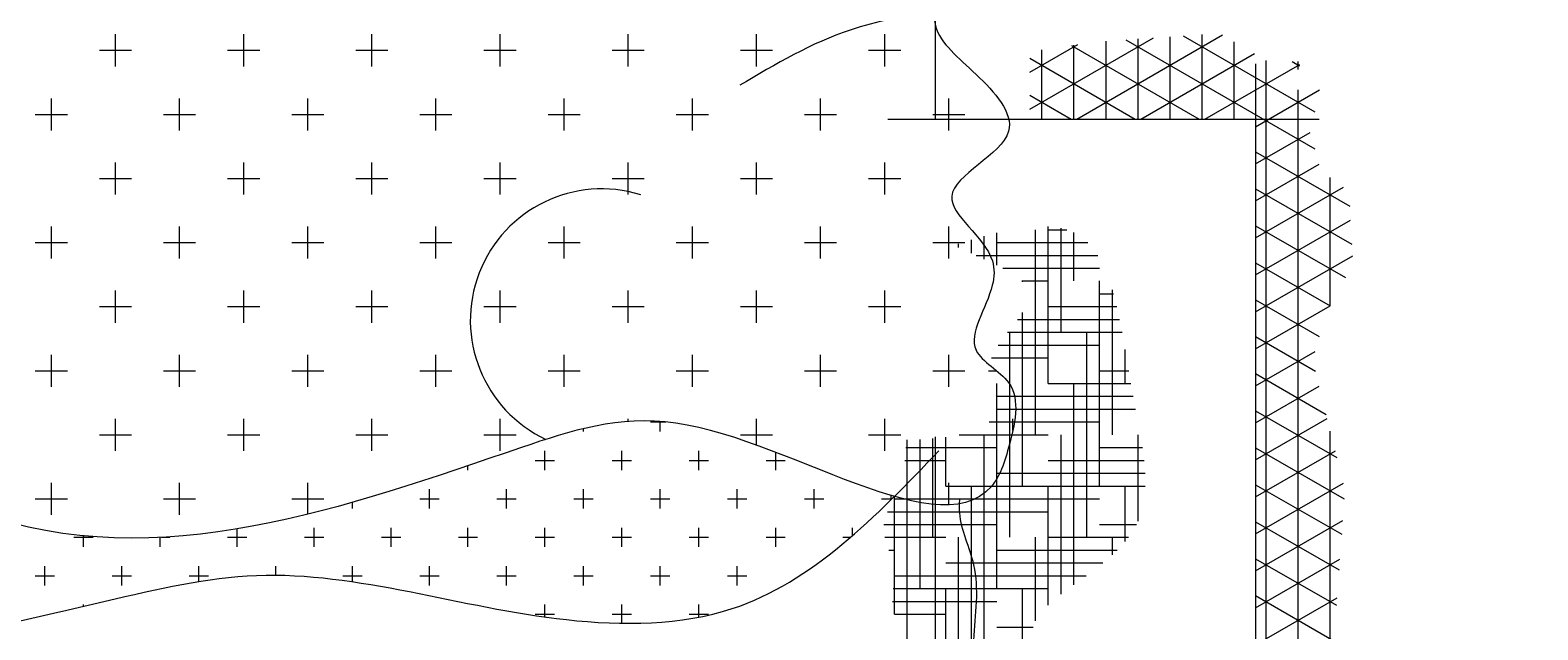
# Model space of a CAD drawing. Units: inches. Extents: x 3731 to 4318, y 1310 to 2388.
# Tile 28 of 57: x 3894 to 3954, y 1882 to 1906. Entities that reach past the tile are written whole.
import ezdxf

# ---------------------------------------------------------------- set-up
doc = ezdxf.new("R2010")
doc.units = ezdxf.units.IN
doc.layers.add('A-ANNO-DIMS', color=2, linetype='Continuous', lineweight=18)
doc.layers.add('A-FURN', color=8, linetype='Continuous', lineweight=13)
doc.styles.get("Standard").update_dxf_attribs({"font": 'arial.ttf'})
doc.dimstyles.get("Standard").update_dxf_attribs({"dimtxt": 0.18, "dimasz": 0.18, "dimexe": 0.18, "dimexo": 0.0625, "dimgap": 0.09, "dimtad": 0, "dimtih": 1, "dimtoh": 1, "dimdec": 4, "dimzin": 0, "dimdsep": 46, "dimtxsty": 'Standard', "dimcen": 0.09, "dimadec": 0, "dimazin": 0, "dimtfac": 1, "dimtdec": 4, "dimtofl": 0, "dimtmove": 0, "dimatfit": 3, "dimfxl": 1, "dimtolj": 1, "dimtzin": 0, "dimarcsym": 0})

# ---------------------------------------------------------------- blocks, each defined once
blk = doc.blocks.new('A$C200C7901')
for p, q in [((2, 1.6055), (2, 2.3334)), ((2.3121, 1.6596), (2.3121, 0.0201)), ((1.9533, 1.6055), (2.3741, 1.6055)), ((1.9533, 1.6055), (2.3741, 1.6055)), ((2, 0.2957), (2, 1.2957)), ((2.0224, 0.9977), (2.0224, 1.1977)), ((2.0224, 0.9977), (2.0224, 1.1977))]:
    blk.add_line(p, q)
at = {"linetype": 'ByBlock'}
for p, q in [((1.2004, 1.657), (1.2004, 1.6883)), ((1.2004, 1.657), (1.2004, 1.6883)), ((1.3254, 1.657), (1.3254, 1.6883)), ((1.3254, 1.657), (1.3254, 1.6883)), ((1.4504, 1.657), (1.4504, 1.6883)), ((1.4504, 1.657), (1.4504, 1.6883)), ((1.5754, 1.657), (1.5754, 1.6883)), ((1.5754, 1.657), (1.5754, 1.6883)), ((1.7004, 1.657), (1.7004, 1.6883)), ((1.7004, 1.657), (1.7004, 1.6883)), ((1.8254, 1.657), (1.8254, 1.6883)), ((1.8254, 1.657), (1.8254, 1.6883)), ((1.9504, 1.657), (1.9504, 1.6883)), ((1.9504, 1.657), (1.9504, 1.6883)), ((2.0919, 1.6152), (2.2125, 1.6848)), ((2.0919, 1.6152), (2.2125, 1.6848)), ((2.0919, 1.6513), (2.1386, 1.6782)), ((2.0919, 1.6513), (2.1386, 1.6782)), ((2.1327, 1.6773), (2.2571, 1.6055)), ((2.1327, 1.6773), (2.2571, 1.6055)), ((2.1349, 1.6055), (2.1349, 1.6777)), ((2.1349, 1.6055), (2.1349, 1.6777)), ((2.1377, 1.6055), (2.2798, 1.6876)), ((2.1377, 1.6055), (2.2798, 1.6876)), ((2.1662, 1.6055), (2.1662, 1.6817)), ((2.1662, 1.6055), (2.1662, 1.6817)), ((2.1854, 1.683), (2.3697, 1.5766)), ((2.1854, 1.683), (2.3697, 1.5766)), ((2.1974, 1.6055), (2.1974, 1.6838)), ((2.1974, 1.6055), (2.1974, 1.6838)), ((2.2287, 1.6055), (2.2287, 1.6859)), ((2.2287, 1.6055), (2.2287, 1.6859)), ((2.2414, 1.6868), (2.3699, 1.6126)), ((2.2414, 1.6868), (2.3699, 1.6126)), ((2.2599, 1.6055), (2.2599, 1.688)), ((2.2599, 1.6055), (2.2599, 1.688)), ((2.2912, 1.6055), (2.2912, 1.6809)), ((2.2912, 1.6055), (2.2912, 1.6809)), ((1.1847, 1.6727), (1.216, 1.6727)), ((1.1847, 1.6727), (1.216, 1.6727)), ((1.3097, 1.6727), (1.341, 1.6727)), ((1.3097, 1.6727), (1.341, 1.6727)), ((1.4347, 1.6727), (1.466, 1.6727)), ((1.4347, 1.6727), (1.466, 1.6727)), ((1.5597, 1.6727), (1.591, 1.6727)), ((1.5597, 1.6727), (1.591, 1.6727)), ((1.6847, 1.6727), (1.716, 1.6727)), ((1.6847, 1.6727), (1.716, 1.6727)), ((1.8097, 1.6727), (1.841, 1.6727)), ((1.8097, 1.6727), (1.841, 1.6727)), ((1.9347, 1.6727), (1.966, 1.6727)), ((1.9347, 1.6727), (1.966, 1.6727)), ((2.0919, 1.6649), (2.1946, 1.6055)), ((2.0919, 1.6649), (2.1946, 1.6055)), ((2.1037, 1.6055), (2.1037, 1.673)), ((2.1037, 1.6055), (2.1037, 1.673)), ((2.2002, 1.6055), (2.3109, 1.6694)), ((2.2002, 1.6055), (2.3109, 1.6694)), ((2.3224, 0.0468), (2.3224, 1.6627)), ((2.3224, 0.0468), (2.3224, 1.6627)), ((2.3476, 1.6616), (2.3547, 1.6575)), ((2.3476, 1.6616), (2.3547, 1.6575)), ((2.3537, 1.6539), (2.3537, 1.6616)), ((2.3537, 1.6539), (2.3537, 1.6616)), ((2.2627, 1.6055), (2.3551, 1.6589)), ((2.2627, 1.6055), (2.3551, 1.6589)), ((2.3121, 1.598), (2.3745, 1.634)), ((2.3121, 1.598), (2.3745, 1.634)), ((2.3537, 0.0056), (2.3537, 1.634)), ((2.3537, 0.0056), (2.3537, 1.634)), ((1.1379, 1.5945), (1.1379, 1.6258)), ((1.1379, 1.5945), (1.1379, 1.6258)), ((1.2629, 1.5945), (1.2629, 1.6258)), ((1.2629, 1.5945), (1.2629, 1.6258)), ((1.3879, 1.5945), (1.3879, 1.6258)), ((1.3879, 1.5945), (1.3879, 1.6258)), ((1.5129, 1.5945), (1.5129, 1.6258)), ((1.5129, 1.5945), (1.5129, 1.6258)), ((1.6379, 1.5945), (1.6379, 1.6258)), ((1.6379, 1.5945), (1.6379, 1.6258)), ((1.7629, 1.5945), (1.7629, 1.6258)), ((1.7629, 1.5945), (1.7629, 1.6258)), ((1.8879, 1.5945), (1.8879, 1.6258)), ((1.8879, 1.5945), (1.8879, 1.6258)), ((2.0129, 1.5945), (2.0129, 1.6258)), ((2.0129, 1.5945), (2.0129, 1.6258)), ((2.0919, 1.6288), (2.1321, 1.6055)), ((2.0919, 1.6288), (2.1321, 1.6055)), ((1.1222, 1.6102), (1.1535, 1.6102)), ((1.1222, 1.6102), (1.1535, 1.6102)), ((1.2472, 1.6102), (1.2785, 1.6102)), ((1.2472, 1.6102), (1.2785, 1.6102)), ((1.3722, 1.6102), (1.4035, 1.6102)), ((1.3722, 1.6102), (1.4035, 1.6102)), ((1.4972, 1.6102), (1.5285, 1.6102)), ((1.4972, 1.6102), (1.5285, 1.6102)), ((1.6222, 1.6102), (1.6535, 1.6102)), ((1.6222, 1.6102), (1.6535, 1.6102)), ((1.7472, 1.6102), (1.7785, 1.6102)), ((1.7472, 1.6102), (1.7785, 1.6102)), ((1.8722, 1.6102), (1.9035, 1.6102)), ((1.8722, 1.6102), (1.9035, 1.6102)), ((1.9972, 1.6102), (2.0285, 1.6102)), ((1.9972, 1.6102), (2.0285, 1.6102)), ((2.3121, 1.5619), (2.3654, 1.5926)), ((2.3121, 1.5619), (2.3654, 1.5926)), ((2.3121, 1.5738), (2.404, 1.5208)), ((2.3121, 1.5738), (2.404, 1.5208)), ((1.2004, 1.532), (1.2004, 1.5633)), ((1.2004, 1.532), (1.2004, 1.5633)), ((1.3254, 1.532), (1.3254, 1.5633)), ((1.3254, 1.532), (1.3254, 1.5633)), ((1.4504, 1.532), (1.4504, 1.5633)), ((1.4504, 1.532), (1.4504, 1.5633)), ((1.5754, 1.532), (1.5754, 1.5633)), ((1.5754, 1.532), (1.5754, 1.5633)), ((1.7004, 1.532), (1.7004, 1.5633)), ((1.7004, 1.532), (1.7004, 1.5633)), ((1.8254, 1.532), (1.8254, 1.5633)), ((1.8254, 1.532), (1.8254, 1.5633)), ((1.9504, 1.532), (1.9504, 1.5633)), ((1.9504, 1.532), (1.9504, 1.5633)), ((2.3121, 1.5258), (2.3739, 1.5615)), ((2.3121, 1.5258), (2.3739, 1.5615)), ((1.1847, 1.5477), (1.216, 1.5477)), ((1.1847, 1.5477), (1.216, 1.5477)), ((1.3097, 1.5477), (1.341, 1.5477)), ((1.3097, 1.5477), (1.341, 1.5477)), ((1.4347, 1.5477), (1.466, 1.5477)), ((1.4347, 1.5477), (1.466, 1.5477)), ((1.5597, 1.5477), (1.591, 1.5477)), ((1.5597, 1.5477), (1.591, 1.5477)), ((1.6847, 1.5477), (1.716, 1.5477)), ((1.6847, 1.5477), (1.716, 1.5477)), ((1.8097, 1.5477), (1.841, 1.5477)), ((1.8097, 1.5477), (1.841, 1.5477)), ((1.9347, 1.5477), (1.966, 1.5477)), ((1.9347, 1.5477), (1.966, 1.5477)), ((2.3849, 1.4236), (2.3849, 1.5486)), ((2.3849, 1.4236), (2.3849, 1.5486)), ((2.3121, 1.4897), (2.3979, 1.5393)), ((2.3121, 1.4897), (2.3979, 1.5393)), ((2.3121, 1.5377), (2.406, 1.4835)), ((2.3121, 1.5377), (2.406, 1.4835)), ((1.1379, 1.4695), (1.1379, 1.5008)), ((1.1379, 1.4695), (1.1379, 1.5008)), ((1.2629, 1.4695), (1.2629, 1.5008)), ((1.2629, 1.4695), (1.2629, 1.5008)), ((1.3879, 1.4695), (1.3879, 1.5008)), ((1.3879, 1.4695), (1.3879, 1.5008)), ((1.5129, 1.4695), (1.5129, 1.5008)), ((1.5129, 1.4695), (1.5129, 1.5008)), ((1.6379, 1.4695), (1.6379, 1.5008)), ((1.6379, 1.4695), (1.6379, 1.5008)), ((1.7629, 1.4695), (1.7629, 1.5008)), ((1.7629, 1.4695), (1.7629, 1.5008)), ((1.8879, 1.4695), (1.8879, 1.5008)), ((1.8879, 1.4695), (1.8879, 1.5008)), ((2.0129, 1.4695), (2.0129, 1.5008)), ((2.0129, 1.4695), (2.0129, 1.5008)), ((2.1099, 1.3477), (2.1099, 1.5009)), ((2.1099, 1.3477), (2.1099, 1.5009)), ((2.3121, 1.4537), (2.4047, 1.5071)), ((2.3121, 1.4537), (2.4047, 1.5071)), ((2.3121, 1.5016), (2.3997, 1.4511)), ((2.3121, 1.5016), (2.3997, 1.4511)), ((1.1222, 1.4852), (1.1535, 1.4852)), ((1.1222, 1.4852), (1.1535, 1.4852)), ((1.2472, 1.4852), (1.2785, 1.4852)), ((1.2472, 1.4852), (1.2785, 1.4852)), ((1.3722, 1.4852), (1.4035, 1.4852)), ((1.3722, 1.4852), (1.4035, 1.4852)), ((1.4972, 1.4852), (1.5285, 1.4852)), ((1.4972, 1.4852), (1.5285, 1.4852)), ((1.6222, 1.4852), (1.6535, 1.4852)), ((1.6222, 1.4852), (1.6535, 1.4852)), ((1.7472, 1.4852), (1.7785, 1.4852)), ((1.7472, 1.4852), (1.7785, 1.4852)), ((1.8722, 1.4852), (1.9035, 1.4852)), ((1.8722, 1.4852), (1.9035, 1.4852)), ((1.9972, 1.4852), (2.0285, 1.4852)), ((1.9972, 1.4852), (2.0285, 1.4852)), ((2.0349, 1.4748), (2.0349, 1.4879)), ((2.0349, 1.4748), (2.0349, 1.4879)), ((2.0474, 1.4691), (2.0474, 1.4915)), ((2.0474, 1.4691), (2.0474, 1.4915)), ((2.0599, 1.4631), (2.0599, 1.4948)), ((2.0599, 1.4631), (2.0599, 1.4948)), ((2.0599, 1.4852), (2.1484, 1.4852)), ((2.0599, 1.4852), (2.1484, 1.4852)), ((2.0974, 1.2977), (2.0974, 1.4977)), ((2.0974, 1.2977), (2.0974, 1.4977)), ((2.1099, 1.4977), (2.1279, 1.4977)), ((2.1099, 1.4977), (2.1279, 1.4977)), ((2.1224, 1.3977), (2.1224, 1.4992)), ((2.1224, 1.3977), (2.1224, 1.4992)), ((2.1349, 1.4477), (2.1349, 1.4949)), ((2.1349, 1.4477), (2.1349, 1.4949)), ((2.0224, 1.4805), (2.0224, 1.4839)), ((2.0224, 1.4805), (2.0224, 1.4839)), ((2.0397, 1.4727), (2.1581, 1.4727)), ((2.0397, 1.4727), (2.1581, 1.4727)), ((2.3121, 1.4176), (2.4067, 1.4721)), ((2.3121, 1.4176), (2.4067, 1.4721)), ((2.0656, 1.4602), (2.1599, 1.4602)), ((2.0656, 1.4602), (2.1599, 1.4602)), ((2.3121, 1.4655), (2.3849, 1.4235)), ((2.3121, 1.4655), (2.3849, 1.4235)), ((2.084, 1.4477), (2.1099, 1.4477)), ((2.084, 1.4477), (2.1099, 1.4477)), ((2.0849, 1.4468), (2.0849, 1.4477)), ((2.0849, 1.4468), (2.0849, 1.4477)), ((2.1599, 1.2477), (2.1599, 1.4477)), ((2.1599, 1.2477), (2.1599, 1.4477)), ((1.2004, 1.407), (1.2004, 1.4383)), ((1.2004, 1.407), (1.2004, 1.4383)), ((1.3254, 1.407), (1.3254, 1.4383)), ((1.3254, 1.407), (1.3254, 1.4383)), ((1.4504, 1.407), (1.4504, 1.4383)), ((1.4504, 1.407), (1.4504, 1.4383)), ((1.5754, 1.407), (1.5754, 1.4383)), ((1.5754, 1.407), (1.5754, 1.4383)), ((1.7004, 1.407), (1.7004, 1.4383)), ((1.7004, 1.407), (1.7004, 1.4383)), ((1.8254, 1.407), (1.8254, 1.4383)), ((1.8254, 1.407), (1.8254, 1.4383)), ((1.9504, 1.407), (1.9504, 1.4383)), ((1.9504, 1.407), (1.9504, 1.4383)), ((2.1599, 1.4352), (2.1735, 1.4352)), ((2.1599, 1.4352), (2.1735, 1.4352)), ((2.1724, 1.2977), (2.1724, 1.439)), ((2.1724, 1.2977), (2.1724, 1.439)), ((2.3121, 1.4294), (2.3741, 1.3937)), ((2.3121, 1.4294), (2.3741, 1.3937)), ((1.1847, 1.4227), (1.216, 1.4227)), ((1.1847, 1.4227), (1.216, 1.4227)), ((1.3097, 1.4227), (1.341, 1.4227)), ((1.3097, 1.4227), (1.341, 1.4227)), ((1.4347, 1.4227), (1.466, 1.4227)), ((1.4347, 1.4227), (1.466, 1.4227)), ((1.5597, 1.4227), (1.591, 1.4227)), ((1.5597, 1.4227), (1.591, 1.4227)), ((1.6847, 1.4227), (1.716, 1.4227)), ((1.6847, 1.4227), (1.716, 1.4227)), ((1.8097, 1.4227), (1.841, 1.4227)), ((1.8097, 1.4227), (1.841, 1.4227)), ((1.9347, 1.4227), (1.966, 1.4227)), ((1.9347, 1.4227), (1.966, 1.4227)), ((2.0849, 1.2477), (2.0849, 1.4171)), ((2.0849, 1.2477), (2.0849, 1.4171)), ((2.1099, 1.4227), (2.1767, 1.4227)), ((2.1099, 1.4227), (2.1767, 1.4227)), ((2.3121, 1.3815), (2.3848, 1.4235)), ((2.3121, 1.3815), (2.3848, 1.4235)), ((2.0703, 1.3977), (2.1819, 1.3977)), ((2.0703, 1.3977), (2.1819, 1.3977)), ((2.0724, 1.1977), (2.0724, 1.3977)), ((2.0724, 1.1977), (2.0724, 1.3977)), ((2.08, 1.4102), (2.1795, 1.4102)), ((2.08, 1.4102), (2.1795, 1.4102)), ((2.1474, 1.1977), (2.1474, 1.3977)), ((2.1474, 1.1977), (2.1474, 1.3977)), ((2.0612, 1.3852), (2.1599, 1.3852)), ((2.0612, 1.3852), (2.1599, 1.3852)), ((2.3121, 1.3934), (2.3703, 1.3598)), ((2.3121, 1.3934), (2.3703, 1.3598)), ((1.1379, 1.3445), (1.1379, 1.3758)), ((1.1379, 1.3445), (1.1379, 1.3758)), ((1.2629, 1.3445), (1.2629, 1.3758)), ((1.2629, 1.3445), (1.2629, 1.3758)), ((1.3879, 1.3445), (1.3879, 1.3758)), ((1.3879, 1.3445), (1.3879, 1.3758)), ((1.5129, 1.3445), (1.5129, 1.3758)), ((1.5129, 1.3445), (1.5129, 1.3758)), ((1.6379, 1.3445), (1.6379, 1.3758)), ((1.6379, 1.3445), (1.6379, 1.3758)), ((1.7629, 1.3445), (1.7629, 1.3758)), ((1.7629, 1.3445), (1.7629, 1.3758)), ((1.8879, 1.3445), (1.8879, 1.3758)), ((1.8879, 1.3445), (1.8879, 1.3758)), ((2.0129, 1.3445), (2.0129, 1.3758)), ((2.0129, 1.3445), (2.0129, 1.3758)), ((2.0545, 1.3727), (2.1099, 1.3727)), ((2.0545, 1.3727), (2.1099, 1.3727)), ((2.1849, 1.3477), (2.1849, 1.3808)), ((2.1849, 1.3477), (2.1849, 1.3808)), ((2.3121, 1.3454), (2.37, 1.3788)), ((2.3121, 1.3454), (2.37, 1.3788)), ((1.1222, 1.3602), (1.1535, 1.3602)), ((1.1222, 1.3602), (1.1535, 1.3602)), ((1.2472, 1.3602), (1.2785, 1.3602)), ((1.2472, 1.3602), (1.2785, 1.3602)), ((1.3722, 1.3602), (1.4035, 1.3602)), ((1.3722, 1.3602), (1.4035, 1.3602)), ((1.4972, 1.3602), (1.5285, 1.3602)), ((1.4972, 1.3602), (1.5285, 1.3602)), ((1.6222, 1.3602), (1.6535, 1.3602)), ((1.6222, 1.3602), (1.6535, 1.3602)), ((1.7472, 1.3602), (1.7785, 1.3602)), ((1.7472, 1.3602), (1.7785, 1.3602)), ((1.8722, 1.3602), (1.9035, 1.3602)), ((1.8722, 1.3602), (1.9035, 1.3602)), ((1.9972, 1.3602), (2.0285, 1.3602)), ((1.9972, 1.3602), (2.0285, 1.3602)), ((2.0515, 1.3602), (2.0599, 1.3602)), ((2.0515, 1.3602), (2.0599, 1.3602)), ((2.1599, 1.3602), (2.1883, 1.3602)), ((2.1599, 1.3602), (2.1883, 1.3602)), ((2.3121, 1.3573), (2.3808, 1.3176)), ((2.3121, 1.3573), (2.3808, 1.3176)), ((2.0599, 1.1477), (2.0599, 1.3477)), ((2.0599, 1.1477), (2.0599, 1.3477)), ((2.1099, 1.3477), (2.1904, 1.3477)), ((2.1099, 1.3477), (2.1904, 1.3477)), ((2.1349, 1.1515), (2.1349, 1.3477)), ((2.1349, 1.1515), (2.1349, 1.3477)), ((2.3121, 1.3093), (2.374, 1.345)), ((2.3121, 1.3093), (2.374, 1.345)), ((2.0599, 1.3352), (2.1926, 1.3352)), ((2.0599, 1.3352), (2.1926, 1.3352)), ((1.2004, 1.282), (1.2004, 1.3133)), ((1.2004, 1.282), (1.2004, 1.3133)), ((1.3254, 1.282), (1.3254, 1.3133)), ((1.3254, 1.282), (1.3254, 1.3133)), ((1.4504, 1.282), (1.4504, 1.3133)), ((1.4504, 1.282), (1.4504, 1.3133)), ((1.5754, 1.282), (1.5754, 1.3133)), ((1.5754, 1.282), (1.5754, 1.3133)), ((1.7004, 1.3106), (1.7004, 1.3133)), ((1.7004, 1.3106), (1.7004, 1.3133)), ((1.7222, 1.3102), (1.7369, 1.3102)), ((1.7222, 1.3102), (1.7369, 1.3102)), ((1.7316, 1.3008), (1.7316, 1.3106)), ((1.7316, 1.3008), (1.7316, 1.3106)), ((1.8254, 1.2876), (1.8254, 1.3133)), ((1.8254, 1.2876), (1.8254, 1.3133)), ((1.9504, 1.282), (1.9504, 1.3133)), ((1.9504, 1.282), (1.9504, 1.3133)), ((2.0524, 1.3102), (2.1599, 1.3102)), ((2.0524, 1.3102), (2.1599, 1.3102)), ((2.0594, 1.3227), (2.195, 1.3227)), ((2.0594, 1.3227), (2.195, 1.3227)), ((2.0754, 1.3017), (2.0754, 1.3133)), ((2.0754, 1.3017), (2.0754, 1.3133)), ((2.3121, 1.3212), (2.3914, 1.2754)), ((2.3121, 1.3212), (2.3914, 1.2754)), ((2.3121, 1.2732), (2.3819, 1.3135)), ((2.3121, 1.2732), (2.3819, 1.3135)), ((1.1847, 1.2977), (1.216, 1.2977)), ((1.1847, 1.2977), (1.216, 1.2977)), ((1.3097, 1.2977), (1.341, 1.2977)), ((1.3097, 1.2977), (1.341, 1.2977)), ((1.4347, 1.2977), (1.466, 1.2977)), ((1.4347, 1.2977), (1.466, 1.2977)), ((1.5597, 1.2977), (1.591, 1.2977)), ((1.5597, 1.2977), (1.591, 1.2977)), ((1.6566, 1.3008), (1.6566, 1.3036)), ((1.6566, 1.3008), (1.6566, 1.3036)), ((1.8097, 1.2977), (1.841, 1.2977)), ((1.8097, 1.2977), (1.841, 1.2977)), ((1.9347, 1.2977), (1.966, 1.2977)), ((1.9347, 1.2977), (1.966, 1.2977)), ((1.9974, 1.1977), (1.9974, 1.2939)), ((1.9974, 1.1977), (1.9974, 1.2939)), ((2.0099, 1.2477), (2.0099, 1.2953)), ((2.0099, 1.2477), (2.0099, 1.2953)), ((2.023, 1.2977), (2.1099, 1.2977)), ((2.023, 1.2977), (2.1099, 1.2977)), ((2.0474, 1.0977), (2.0474, 1.2977)), ((2.0474, 1.0977), (2.0474, 1.2977)), ((2.0597, 1.2977), (2.0744, 1.2977)), ((2.0597, 1.2977), (2.0744, 1.2977)), ((2.1224, 1.1421), (2.1224, 1.2977)), ((2.1224, 1.1421), (2.1224, 1.2977)), ((2.1974, 1.2135), (2.1974, 1.2977)), ((2.1974, 1.2135), (2.1974, 1.2977)), ((2.3849, 1.0607), (2.3849, 1.3013)), ((2.3849, 1.0607), (2.3849, 1.3013)), ((1.6191, 1.2633), (1.6191, 1.282)), ((1.6191, 1.2633), (1.6191, 1.282)), ((1.6941, 1.2633), (1.6941, 1.282)), ((1.6941, 1.2633), (1.6941, 1.282)), ((1.7691, 1.2633), (1.7691, 1.282)), ((1.7691, 1.2633), (1.7691, 1.282)), ((1.8441, 1.2633), (1.8441, 1.2806)), ((1.8441, 1.2633), (1.8441, 1.2806)), ((1.9711, 1.2852), (2.0599, 1.2852)), ((1.9711, 1.2852), (2.0599, 1.2852)), ((1.9724, 1.0977), (1.9724, 1.2927)), ((1.9724, 1.0977), (1.9724, 1.2927)), ((1.9849, 1.1477), (1.9849, 1.293)), ((1.9849, 1.1477), (1.9849, 1.293)), ((2.1599, 1.2852), (2.2018, 1.2852)), ((2.1599, 1.2852), (2.2018, 1.2852)), ((2.3121, 1.2851), (2.3985, 1.2352)), ((2.3121, 1.2851), (2.3985, 1.2352)), ((2.3121, 1.2371), (2.3898, 1.282)), ((2.3121, 1.2371), (2.3898, 1.282)), ((1.5441, 1.2633), (1.5441, 1.2675)), ((1.5441, 1.2633), (1.5441, 1.2675)), ((1.6097, 1.2727), (1.6285, 1.2727)), ((1.6097, 1.2727), (1.6285, 1.2727)), ((1.6847, 1.2727), (1.7035, 1.2727)), ((1.6847, 1.2727), (1.7035, 1.2727)), ((1.7597, 1.2727), (1.7785, 1.2727)), ((1.7597, 1.2727), (1.7785, 1.2727)), ((1.8347, 1.2727), (1.8535, 1.2727)), ((1.8347, 1.2727), (1.8535, 1.2727)), ((1.97, 1.2727), (2.0099, 1.2727)), ((1.97, 1.2727), (2.0099, 1.2727)), ((2.1099, 1.2727), (2.2034, 1.2727)), ((2.1099, 1.2727), (2.2034, 1.2727)), ((1.1379, 1.2195), (1.1379, 1.2508)), ((1.1379, 1.2195), (1.1379, 1.2508)), ((1.2629, 1.2195), (1.2629, 1.2508)), ((1.2629, 1.2195), (1.2629, 1.2508)), ((1.3879, 1.2202), (1.3879, 1.2508)), ((1.3879, 1.2202), (1.3879, 1.2508)), ((2.0129, 1.2293), (2.0129, 1.2508)), ((2.0129, 1.2293), (2.0129, 1.2508)), ((2.0599, 1.2602), (2.2044, 1.2602)), ((2.0599, 1.2602), (2.2044, 1.2602)), ((2.3121, 1.2011), (2.3976, 1.2504)), ((2.3121, 1.2011), (2.3976, 1.2504)), ((1.1222, 1.2352), (1.1535, 1.2352)), ((1.1222, 1.2352), (1.1535, 1.2352)), ((1.2472, 1.2352), (1.2785, 1.2352)), ((1.2472, 1.2352), (1.2785, 1.2352)), ((1.3722, 1.2352), (1.4035, 1.2352)), ((1.3722, 1.2352), (1.4035, 1.2352)), ((1.4972, 1.2352), (1.516, 1.2352)), ((1.4972, 1.2352), (1.516, 1.2352)), ((1.5066, 1.2258), (1.5066, 1.2445)), ((1.5066, 1.2258), (1.5066, 1.2445)), ((1.5722, 1.2352), (1.591, 1.2352)), ((1.5722, 1.2352), (1.591, 1.2352)), ((1.5816, 1.2258), (1.5816, 1.2445)), ((1.5816, 1.2258), (1.5816, 1.2445)), ((1.6472, 1.2352), (1.666, 1.2352)), ((1.6472, 1.2352), (1.666, 1.2352)), ((1.6566, 1.2258), (1.6566, 1.2445)), ((1.6566, 1.2258), (1.6566, 1.2445)), ((1.7222, 1.2352), (1.741, 1.2352)), ((1.7222, 1.2352), (1.741, 1.2352)), ((1.7316, 1.2258), (1.7316, 1.2445)), ((1.7316, 1.2258), (1.7316, 1.2445)), ((1.7972, 1.2352), (1.816, 1.2352)), ((1.7972, 1.2352), (1.816, 1.2352)), ((1.8066, 1.2258), (1.8066, 1.2445)), ((1.8066, 1.2258), (1.8066, 1.2445)), ((1.8722, 1.2352), (1.891, 1.2352)), ((1.8722, 1.2352), (1.891, 1.2352)), ((1.8816, 1.2258), (1.8816, 1.2445)), ((1.8816, 1.2258), (1.8816, 1.2445)), ((1.9472, 1.2352), (1.9574, 1.2352)), ((1.9472, 1.2352), (1.9574, 1.2352)), ((1.9566, 1.2344), (1.9566, 1.2385)), ((1.9566, 1.2344), (1.9566, 1.2385)), ((1.9599, 1.1228), (1.9599, 1.2373)), ((1.9599, 1.1228), (1.9599, 1.2373)), ((1.9599, 1.2352), (2.1599, 1.2352)), ((1.9599, 1.2352), (2.1599, 1.2352)), ((2, 1.2352), (2.0285, 1.2352)), ((2, 1.2352), (2.0285, 1.2352)), ((2.0099, 1.2477), (2.2045, 1.2477)), ((2.0099, 1.2477), (2.2045, 1.2477)), ((2.0349, 1.0477), (2.0349, 1.2477)), ((2.0349, 1.0477), (2.0349, 1.2477)), ((2.1099, 1.1315), (2.1099, 1.2477)), ((2.1099, 1.1315), (2.1099, 1.2477)), ((2.1849, 1.1935), (2.1849, 1.2477)), ((2.1849, 1.1935), (2.1849, 1.2477)), ((2.3121, 1.249), (2.396, 1.2006)), ((2.3121, 1.249), (2.396, 1.2006)), ((1.4316, 1.2258), (1.4316, 1.2318)), ((1.4316, 1.2258), (1.4316, 1.2318)), ((1.953, 1.2227), (2.1099, 1.2227)), ((1.953, 1.2227), (2.1099, 1.2227)), ((1.3191, 1.1883), (1.3191, 1.2059)), ((1.3191, 1.1883), (1.3191, 1.2059)), ((1.3941, 1.1883), (1.3941, 1.207)), ((1.3941, 1.1883), (1.3941, 1.207)), ((1.4691, 1.1883), (1.4691, 1.207)), ((1.4691, 1.1883), (1.4691, 1.207)), ((1.5441, 1.1883), (1.5441, 1.207)), ((1.5441, 1.1883), (1.5441, 1.207)), ((1.6191, 1.1883), (1.6191, 1.207)), ((1.6191, 1.1883), (1.6191, 1.207)), ((1.6941, 1.1883), (1.6941, 1.207)), ((1.6941, 1.1883), (1.6941, 1.207)), ((1.7691, 1.1883), (1.7691, 1.207)), ((1.7691, 1.1883), (1.7691, 1.207)), ((1.8441, 1.1883), (1.8441, 1.207)), ((1.8441, 1.1883), (1.8441, 1.207)), ((1.9191, 1.1995), (1.9191, 1.207)), ((1.9191, 1.1995), (1.9191, 1.207)), ((1.9495, 1.2102), (2.0599, 1.2102)), ((1.9495, 1.2102), (2.0599, 1.2102)), ((2.1599, 1.2102), (2.1959, 1.2102)), ((2.1599, 1.2102), (2.1959, 1.2102)), ((2.3121, 1.165), (2.397, 1.214)), ((2.3121, 1.165), (2.397, 1.214)), ((2.3121, 1.2129), (2.3935, 1.166)), ((2.3121, 1.2129), (2.3935, 1.166)), ((1.1597, 1.1977), (1.1785, 1.1977)), ((1.1597, 1.1977), (1.1785, 1.1977)), ((1.1691, 1.1883), (1.1691, 1.1991)), ((1.1691, 1.1883), (1.1691, 1.1991)), ((1.2441, 1.1883), (1.2441, 1.1976)), ((1.2441, 1.1883), (1.2441, 1.1976)), ((1.2452, 1.1977), (1.2535, 1.1977)), ((1.2452, 1.1977), (1.2535, 1.1977)), ((1.3097, 1.1977), (1.3285, 1.1977)), ((1.3097, 1.1977), (1.3285, 1.1977)), ((1.3847, 1.1977), (1.4035, 1.1977)), ((1.3847, 1.1977), (1.4035, 1.1977)), ((1.4597, 1.1977), (1.4785, 1.1977)), ((1.4597, 1.1977), (1.4785, 1.1977)), ((1.5347, 1.1977), (1.5535, 1.1977)), ((1.5347, 1.1977), (1.5535, 1.1977)), ((1.6097, 1.1977), (1.6285, 1.1977)), ((1.6097, 1.1977), (1.6285, 1.1977)), ((1.6847, 1.1977), (1.7035, 1.1977)), ((1.6847, 1.1977), (1.7035, 1.1977)), ((1.7597, 1.1977), (1.7785, 1.1977)), ((1.7597, 1.1977), (1.7785, 1.1977)), ((1.8347, 1.1977), (1.8535, 1.1977)), ((1.8347, 1.1977), (1.8535, 1.1977)), ((1.9097, 1.1977), (1.917, 1.1977)), ((1.9097, 1.1977), (1.917, 1.1977)), ((1.9506, 1.1977), (2.0099, 1.1977)), ((1.9506, 1.1977), (2.0099, 1.1977)), ((2.0974, 1.1161), (2.0974, 1.1977)), ((2.0974, 1.1161), (2.0974, 1.1977)), ((2.1099, 1.1977), (2.1882, 1.1977)), ((2.1099, 1.1977), (2.1882, 1.1977)), ((2.1724, 1.1807), (2.1724, 1.1977)), ((2.1724, 1.1807), (2.1724, 1.1977)), ((1.9545, 1.1852), (1.9599, 1.1852)), ((1.9545, 1.1852), (1.9599, 1.1852)), ((2.0599, 1.1852), (2.1772, 1.1852)), ((2.0599, 1.1852), (2.1772, 1.1852)), ((2.3121, 1.1768), (2.3909, 1.1314)), ((2.3121, 1.1768), (2.3909, 1.1314)), ((2.3121, 1.1289), (2.3942, 1.1763)), ((2.3121, 1.1289), (2.3942, 1.1763)), ((1.1316, 1.1508), (1.1316, 1.1695)), ((1.1316, 1.1508), (1.1316, 1.1695)), ((1.2066, 1.1508), (1.2066, 1.1695)), ((1.2066, 1.1508), (1.2066, 1.1695)), ((1.2816, 1.1547), (1.2816, 1.1695)), ((1.2816, 1.1547), (1.2816, 1.1695)), ((1.3566, 1.1608), (1.3566, 1.1695)), ((1.3566, 1.1608), (1.3566, 1.1695)), ((1.4316, 1.1544), (1.4316, 1.1695)), ((1.4316, 1.1544), (1.4316, 1.1695)), ((1.5066, 1.1508), (1.5066, 1.1695)), ((1.5066, 1.1508), (1.5066, 1.1695)), ((1.5816, 1.1508), (1.5816, 1.1695)), ((1.5816, 1.1508), (1.5816, 1.1695)), ((1.6566, 1.1508), (1.6566, 1.1695)), ((1.6566, 1.1508), (1.6566, 1.1695)), ((1.7316, 1.1508), (1.7316, 1.1695)), ((1.7316, 1.1508), (1.7316, 1.1695)), ((1.8066, 1.1508), (1.8066, 1.1695)), ((1.8066, 1.1508), (1.8066, 1.1695)), ((2.0099, 1.1727), (2.1631, 1.1727)), ((2.0099, 1.1727), (2.1631, 1.1727)), ((1.1222, 1.1602), (1.141, 1.1602)), ((1.1222, 1.1602), (1.141, 1.1602)), ((1.1972, 1.1602), (1.216, 1.1602)), ((1.1972, 1.1602), (1.216, 1.1602)), ((1.2722, 1.1602), (1.291, 1.1602)), ((1.2722, 1.1602), (1.291, 1.1602)), ((1.4222, 1.1602), (1.441, 1.1602)), ((1.4222, 1.1602), (1.441, 1.1602)), ((1.4972, 1.1602), (1.516, 1.1602)), ((1.4972, 1.1602), (1.516, 1.1602)), ((1.5722, 1.1602), (1.591, 1.1602)), ((1.5722, 1.1602), (1.591, 1.1602)), ((1.6472, 1.1602), (1.666, 1.1602)), ((1.6472, 1.1602), (1.666, 1.1602)), ((1.7222, 1.1602), (1.741, 1.1602)), ((1.7222, 1.1602), (1.741, 1.1602)), ((1.7972, 1.1602), (1.816, 1.1602)), ((1.7972, 1.1602), (1.816, 1.1602)), ((1.9585, 1.1477), (2.1099, 1.1477)), ((1.9585, 1.1477), (2.1099, 1.1477)), ((1.9599, 1.1602), (2.1468, 1.1602)), ((1.9599, 1.1602), (2.1468, 1.1602)), ((2.0099, 0.9477), (2.0099, 1.1477)), ((2.0099, 0.9477), (2.0099, 1.1477)), ((2.0849, 0.9477), (2.0849, 1.1477)), ((2.0849, 0.9477), (2.0849, 1.1477)), ((1.1691, 1.1303), (1.1691, 1.132)), ((1.1691, 1.1303), (1.1691, 1.132)), ((1.6191, 1.1201), (1.6191, 1.132)), ((1.6191, 1.1201), (1.6191, 1.132)), ((1.6941, 1.1139), (1.6941, 1.132)), ((1.6941, 1.1139), (1.6941, 1.132)), ((1.7691, 1.1198), (1.7691, 1.132)), ((1.7691, 1.1198), (1.7691, 1.132)), ((1.9581, 1.1352), (2.0599, 1.1352)), ((1.9581, 1.1352), (2.0599, 1.1352)), ((2.3121, 1.1408), (2.3884, 1.0967)), ((2.3121, 1.1408), (2.3884, 1.0967)), ((2.3121, 1.0928), (2.3915, 1.1386)), ((2.3121, 1.0928), (2.3915, 1.1386)), ((1.6097, 1.1227), (1.6285, 1.1227)), ((1.6097, 1.1227), (1.6285, 1.1227)), ((1.6847, 1.1227), (1.7035, 1.1227)), ((1.6847, 1.1227), (1.7035, 1.1227)), ((1.7597, 1.1227), (1.7785, 1.1227)), ((1.7597, 1.1227), (1.7785, 1.1227)), ((1.9599, 1.1227), (2.0099, 1.1227)), ((1.9599, 1.1227), (2.0099, 1.1227)), ((2.0599, 1.1102), (2.0951, 1.1102)), ((2.0599, 1.1102), (2.0951, 1.1102))]:
    blk.add_line(p, q, dxfattribs=at)
blk.add_arc((1.6746, 1.4093), 0.1282, 72.7909, 244.8695, dxfattribs=at)
blk.add_arc((1.6746, 1.4093), 0.1282, 72.7909, 244.8695, dxfattribs=at)
for points, knots in [([(0.4485, 1.7835), (0.4321, 1.7496), (0.4062, 1.6964), (0.49, 1.6713), (0.4719, 1.5969), (0.4123, 1.592), (0.4233, 1.5337), (0.4954, 1.5086), (0.4012, 1.4738), (0.3253, 1.4306), (0.4113, 1.3764), (0.3688, 1.3065), (0.5579, 1.2663), (0.741, 1.4533), (1.1127, 1.1109), (1.4811, 1.2478), (1.7885, 1.3492), (2.0357, 1.1637), (2.0748, 1.2974), (2.0876, 1.349), (2.0192, 1.3805), (2.0564, 1.4298), (2.0588, 1.4846), (1.9759, 1.5349), (2.1004, 1.5845), (2.0397, 1.6519), (1.971, 1.7053), (2.1104, 1.8981), (1.5946, 1.7967), (1.2448, 1.7472), (0.8129, 1.7935), (0.4953, 1.8548), (0.4582, 1.7983), (0.4485, 1.7835)], [0, 0, 0, 0, 88.420092, 139.08588, 204.302936, 239.695496, 287.801042, 327.365471, 412.960499, 463.626286, 552.059846, 584.668336, 662.614915, 940.993281, 1309.926334, 1844.022653, 1996.276242, 2316.43048, 2341.441004, 2404.707416, 2449.463774, 2514.680778, 2538.40571, 2613.031547, 2697.13096, 2760.903931, 2822.692699, 2945.47, 3215.060018, 3725.584917, 4361.974444, 4504.671998, 4555.32777, 4555.32777, 4555.32777, 4555.32777]), ([(0.4856, 1.3429), (0.5504, 1.3182), (0.6715, 1.2721), (0.8374, 1.0498), (1.1164, 1.1183), (1.3878, 1.1816), (1.5888, 1.1102), (1.8403, 1.1127), (1.9415, 1.2178), (2.0032, 1.2819)], [0, 0, 0, 0, 205.411753, 383.654933, 772.067458, 921.644661, 1226.793228, 1388.983508, 1642.292305, 1642.292305, 1642.292305, 1642.292305])]:
    blk.add_open_spline(points, degree=3, knots=knots)
for points, knots in [([(1.996, 1.7104), (1.9692, 1.7057), (1.9025, 1.6938), (1.844, 1.6592), (1.809, 1.6385)], [0, 0, 0, 0, 81.132613, 201.738644, 201.738644, 201.738644, 201.738644]), ([(1.996, 1.7104), (1.9692, 1.7057), (1.9025, 1.6938), (1.844, 1.6592), (1.809, 1.6385)], [0, 0, 0, 0, 81.132613, 201.738644, 201.738644, 201.738644, 201.738644]), ([(0.473, 1.2954), (0.4739, 1.2781), (0.4755, 1.2477), (0.5032, 1.2084), (0.4801, 1.1701), (0.4928, 1.1255), (0.4674, 1.0912), (0.4579, 1.0351), (0.501, 0.9724), (0.4311, 0.8832), (0.4902, 0.8637), (0.4843, 0.8288), (0.4774, 0.7906), (0.4625, 0.7457), (0.459, 0.6999), (0.4816, 0.6664), (0.4748, 0.625), (0.4791, 0.5889), (0.4533, 0.5528), (0.4738, 0.5004), (0.4658, 0.4502), (0.4696, 0.3946), (0.4189, 0.3935), (0.4493, 0.3684), (0.4694, 0.3857), (0.4922, 0.3576), (0.5297, 0.3262), (0.5917, 0.3353), (0.6454, 0.3754), (0.7083, 0.3741), (0.7643, 0.3328), (0.826, 0.346), (0.925, 0.3388), (1.0353, 0.3593), (1.1561, 0.3744), (1.2477, 0.3154), (1.3302, 0.3474), (1.4086, 0.3512), (1.5217, 0.3878), (1.6362, 0.3176), (1.7682, 0.3285), (1.8402, 0.3019), (1.9071, 0.3529), (1.9647, 0.3412), (2.0795, 0.2948), (2.0472, 0.3498), (2.0343, 0.3772), (2.0435, 0.43), (2.0109, 0.5782), (2.0746, 0.4643), (2.0805, 0.584), (2.0084, 0.5979), (2.0343, 0.6846), (2.0344, 0.746), (2.0293, 0.8096), (2.0489, 0.8545), (2.0652, 0.9218), (1.9842, 0.9297), (2.0007, 1.0162), (2.0367, 1.0585), (2.0367, 1.1102), (2.0457, 1.1647), (2.0226, 1.2084), (2.0234, 1.2306), (2.0236, 1.2352)], [0, 0, 0, 0, 51.660678, 90.967412, 128.902454, 170.303599, 219.852997, 247.834962, 336.321557, 429.35469, 458.821847, 477.222321, 524.135809, 581.038434, 617.839381, 657.146115, 693.947125, 740.178081, 760.753248, 820.731705, 885.133458, 928.777044, 953.563729, 976.574207, 995.553042, 1018.563482, 1064.584401, 1147.951297, 1174.787598, 1266.851571, 1308.018447, 1377.066427, 1441.511314, 1608.245014, 1714.11869, 1792.771707, 1913.247991, 1954.931389, 2029.864445, 2259.189419, 2305.221512, 2429.507982, 2456.344283, 2543.92595, 2627.925037, 2662.96218, 2687.736879, 2719.937755, 2839.540991, 2875.47895, 2953.681041, 2993.270313, 3066.872333, 3154.395764, 3200.397042, 3248.426375, 3312.828127, 3347.881398, 3444.484026, 3481.577522, 3518.665244, 3592.267265, 3644.719162, 3658.519501, 3658.519501, 3658.519501, 3658.519501])]:
    blk.add_open_spline(points, degree=3, knots=knots, dxfattribs=at)
blk = doc.blocks.new('*D45')
at = {"layer": 'A-ANNO-DIMS', "color": 0, "lineweight": -2, "transparency": 16777216}
for p, q in [((3969.146, 1934.382), (3731.412, 1934.382)), ((3731.592, 1934.202), (3731.592, 1904.563)), ((3731.592, 1874.562), (3731.592, 1904.2)), ((3969.146, 1874.382), (3731.412, 1874.382))]:
    blk.add_line(p, q, dxfattribs=at)
at = {"layer": 'A-ANNO-DIMS', "color": 0, "transparency": 16777216}
for points in [[(3731.562, 1934.202), (3731.622, 1934.202), (3731.592, 1934.382)], [(3731.562, 1874.562), (3731.622, 1874.562), (3731.592, 1874.382)]]:
    blk.add_solid(points, dxfattribs=at)
at = {"layer": 'Defpoints', "color": 0, "transparency": 16777216}
for p in [(3731.592, 1934.382), (3969.209, 1934.382), (3969.209, 1874.382)]:
    blk.add_point(p, dxfattribs=at)
at = {"layer": 'A-ANNO-DIMS', "color": 0, "transparency": 16777216, "insert": (3731.592, 1904.382), "char_height": 0.18, "attachment_point": 5}
blk.add_mtext('\\A1;60', dxfattribs=at)

msp = doc.modelspace()

# ---------------------------------------------------------------- block references
at = {"layer": 'A-FURN', "xscale": 41.1071563136412, "yscale": 41.1071563136412, "zscale": 41.1071563136412}
msp.add_blockref('A$C200C7901', (3848.004, 1836.625), dxfattribs=at)

# ---------------------------------------------------------------- dimensions: what is measured, and where the dimension line sits
at = {"layer": 'A-ANNO-DIMS'}
dim = msp.add_linear_dim(base=(3731.592, 1934.382), p1=(3969.209, 1874.382), p2=(3969.209, 1934.382), angle=90, dimstyle='Standard', override={"dimdec": 0, "dimlfac": 1, "dimrnd": 0, "dimzin": 0, "dimdsep": 46, "dimlunit": 2}, dxfattribs=at)
dim.commit()
dim.dimension.update_dxf_attribs({"geometry": '*D45', "text_midpoint": (3731.592, 1904.382)})

doc.saveas('drawing.dxf')
